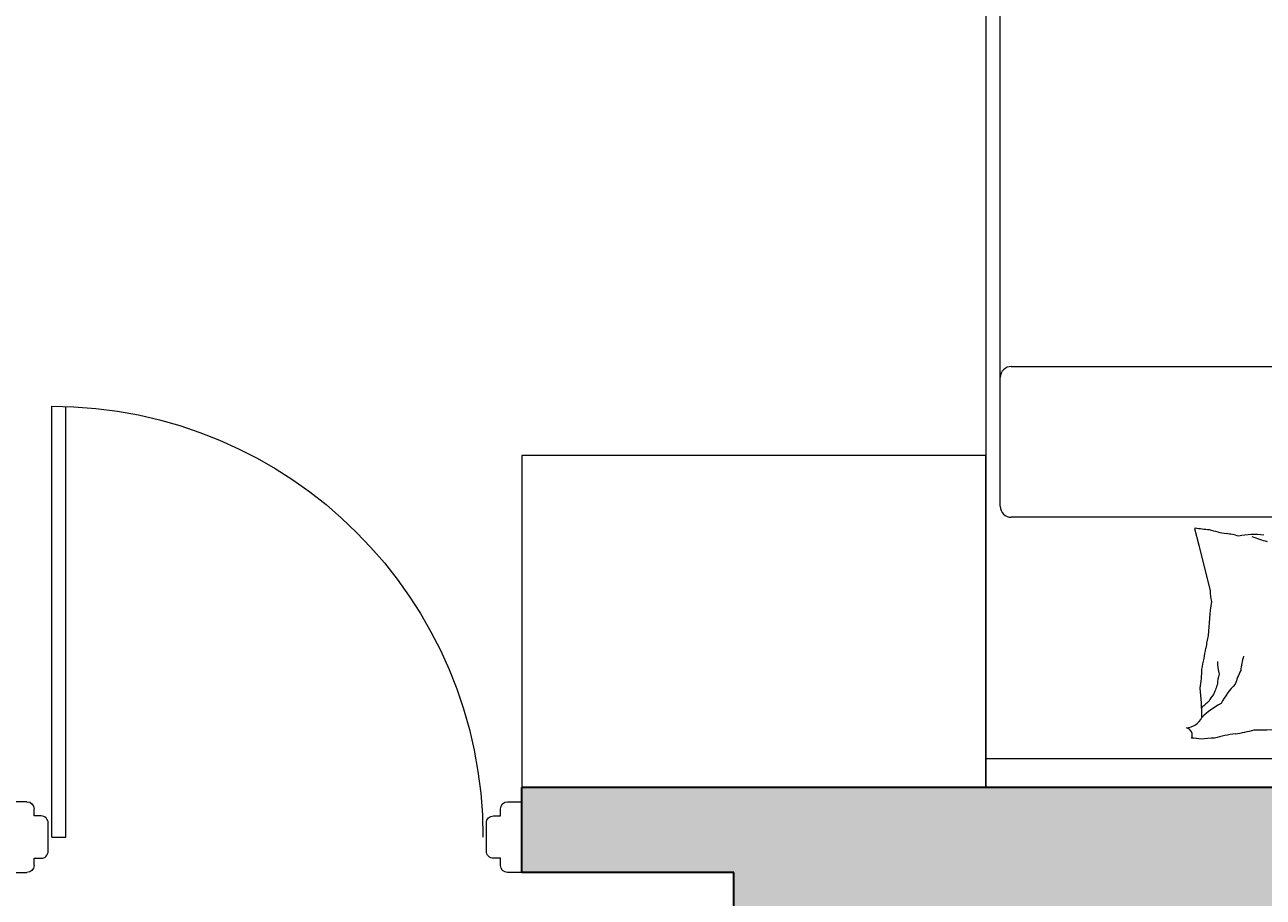
# Model space of a CAD drawing. Units: inches. Extents: x 84 to 1044, y -280 to 906.
# Tile 78 of 105: x 645 to 733, y 512 to 574. Entities that reach past the tile are written whole.
import ezdxf

# ---------------------------------------------------------------- set-up
doc = ezdxf.new("R2010")
doc.units = ezdxf.units.IN
for name, color, linetype, lineweight in [('00 FURNITURE', 15, 'Continuous', 15), ('A-ANNO-DIMS', 2, 'Continuous', 18), ('A-DOOR', 4, 'Continuous', 18), ('A-FURN', 8, 'Continuous', 15), ('WALL', 250, 'Continuous', 35)]:
    doc.layers.add(name, color=color, linetype=linetype, lineweight=lineweight)
doc.layers.add('A-WALL-PATT', color=251, linetype='Continuous', lineweight=9, true_color=0x636466)
doc.styles.get("Standard").update_dxf_attribs({"font": 'arial.ttf'})
doc.dimstyles.get("Standard").update_dxf_attribs({"dimtxt": 0.18, "dimasz": 0.18, "dimexe": 0.18, "dimexo": 0.0625, "dimgap": 0.09, "dimtad": 0, "dimtih": 1, "dimtoh": 1, "dimdec": 4, "dimzin": 0, "dimdsep": 46, "dimtxsty": 'Standard', "dimcen": 0.09, "dimadec": 0, "dimazin": 0, "dimtfac": 1, "dimtdec": 4, "dimtofl": 0, "dimtmove": 0, "dimatfit": 3, "dimfxl": 1, "dimtolj": 1, "dimtzin": 0, "dimarcsym": 0})

# ---------------------------------------------------------------- blocks, each defined once
blk = doc.blocks.new('DDD')
at = {"layer": '00 FURNITURE'}
for p, q in [((-12579.773, -15859.529), (-12579.773, -15829.045)), ((-12578.773, -15859.529), (-12578.773, -15829.029)), ((-12612.023, -15857.029), (-12612.023, -15862.029)), ((-12611.023, -15857.029), (-12612.023, -15857.029)), ((-12577.023, -15857.029), (-12576.023, -15857.029)), ((-12576.023, -15857.029), (-12576.023, -15862.029)), ((-12610.523, -15858.029), (-12610.523, -15857.529)), ((-12577.523, -15858.029), (-12577.523, -15857.529)), ((-12578.773, -15859.529), (-12579.773, -15859.529)), ((-12610.523, -15861.529), (-12610.523, -15861.029)), ((-12577.523, -15861.529), (-12577.523, -15861.029)), ((-12612.023, -15862.029), (-12611.023, -15862.029)), ((-12576.023, -15862.029), (-12577.023, -15862.029))]:
    blk.add_line(p, q, dxfattribs=at)
for points in [[(-12610.523, -15861.029), (-12610.023, -15861.029, 0.414214), (-12609.523, -15860.529), (-12609.523, -15858.529, 0.414214), (-12610.023, -15858.029), (-12610.523, -15858.029)], [(-12577.523, -15861.029), (-12578.023, -15861.029, -0.414214), (-12578.523, -15860.529), (-12578.523, -15858.529, -0.414214), (-12578.023, -15858.029), (-12577.523, -15858.029)]]:
    blk.add_lwpolyline(points, format="xyb", dxfattribs=at)
for centre, radius, start, end in [((-12578.773, -15859.529), 30.5, 90, 180), ((-12611.023, -15857.529), 0.5, 0, 90), ((-12577.023, -15857.529), 0.5, 90, 180), ((-12611.023, -15861.529), 0.5, 270, 0), ((-12577.023, -15861.529), 0.5, 180, 270)]:
    blk.add_arc(centre, radius, start, end, dxfattribs=at)
blk = doc.blocks.new('BED-DOUBLE-NIGHTSTANDS')
for p, q in [((33.845, 19.919), (33.845, 77.08)), ((34.629, 29.814), (88.271, 29.814)), ((85.85, 19.136), (34.629, 19.136)), ((47.596, 18.345), (47.89, 17.169)), ((47.89, 17.169), (48.699, 13.934)), ((32.834, 2.051), (111.174, 2.051))]:
    blk.add_line(p, q)
for points in [[(32.834, 78.34), (32.834, 0), (111.174, 0), (111.174, 78.34)], [(0.004, 23.502), (0.004, 0), (32.834, 0), (32.834, 23.502)]]:
    blk.add_lwpolyline(points, close=True)
for centre, radius, start, end in [((34.629, 29.03), 0.783, 90, 180), ((34.629, 19.919), 0.783, 180, 270), ((47.598, 18.38), 0.0359, 265.91706, 14.04494), ((49.381, 28.85), 10.605, 260.5159, 265.91706), ((51.314, 26.856), 8.996, 252.61359, 260.5159), ((49.306, 13.323), 4.69, 72.61359, 83.56595), ((51.852, 12.199), 5.715, 83.56595, 101.55856), ((61.275, 45.057), 28.934, 250.57202, 252.80178), ((74.329, 9.574), 25.804, 171.99495, 177.33512), ((51.349, 13.811), 2.652, 177.33512, 194.04519), ((60.693, 8.149), 12.422, 167.80162, 171.99495), ((14.336, 15.691), 34.549, 347.80162, 350.31563), ((52.799, 8.936), 3.585, 180, 194.68511), ((56.308, 7.745), 5.482, 163.48502, 174.36887), ((40.115, 8.39), 7.99, 350.31563, 0), ((51.414, 7.319), 2.2, 161.2201, 180), ((55.72, 5.76), 5.482, 152.60117, 163.48502), ((28.84, 4.955), 19.265, 0, 6.23236), ((56.689, 4.327), 8.052, 158.18508, 161.2201), ((54.334, 3.436), 5.482, 134.90238, 152.60117), ((50.464, 5.22), 2.061, 138.55709, 154.64488), ((54.414, 4.384), 5.918, 154.64488, 158.18508), ((50.684, 3.264), 3.52, 126.26407, 138.55709), ((51.973, 1.083), 5.482, 117.20359, 134.90238), ((46.913, 5.566), 1.339, 274.40021, 333.41948), ((46.915, 3.726), 0.514, 333.41948, 78.72762), ((52.232, -7.993), 11.938, 98.43719, 105.74398), ((49.235, 13.221), 9.489, 277.54685, 285.74398), ((51.809, 30.83), 26.741, 270, 277.54685), ((47.375, -0.045), 3.541, 78.72762, 90), ((48.993, -2.815), 6.312, 90, 98.43719)]:
    blk.add_arc(centre, radius, start, end)
blk = doc.blocks.new('*D62')
at = {"layer": 'A-ANNO-DIMS', "color": 0, "lineweight": -2, "transparency": 16777216}
for p, q in [((203.179, 709.183), (203.179, 905.9)), ((896.074, 400.183), (896.074, 905.9)), ((203.359, 905.72), (549.232, 905.72)), ((895.894, 905.72), (550.021, 905.72))]:
    blk.add_line(p, q, dxfattribs=at)
at = {"layer": 'A-ANNO-DIMS', "color": 0, "transparency": 16777216}
for points in [[(203.359, 905.75), (203.359, 905.69), (203.179, 905.72)], [(895.894, 905.75), (895.894, 905.69), (896.074, 905.72)]]:
    blk.add_solid(points, dxfattribs=at)
at = {"layer": 'Defpoints', "color": 0, "transparency": 16777216}
for p in [(896.074, 905.72), (203.179, 709.12), (896.074, 400.12)]:
    blk.add_point(p, dxfattribs=at)
at = {"layer": 'A-ANNO-DIMS', "color": 0, "transparency": 16777216, "insert": (549.627, 905.72), "char_height": 0.18, "attachment_point": 5}
blk.add_mtext('\\A1;692.9', dxfattribs=at)

msp = doc.modelspace()

# ---------------------------------------------------------------- hatches: boundary and pattern name
at = {"layer": 'A-WALL-PATT', "transparency": 33554597}
h = msp.add_hatch(color=256, dxfattribs=at)
h.dxf.hatch_style = 1
h.paths.add_polyline_path([(671.074, 100.12), (647.074, 100.12), (647.074, 160.12), (641.074, 160.12), (620.824, 160.12), (620.824, 151.12), (638.074, 151.12), (638.074, 91.12), (671.074, 91.12)])
h.paths.add_polyline_path([(791.074, 100.12), (743.074, 100.12), (743.074, 91.12), (791.074, 91.12)])
h.paths.add_polyline_path([(896.074, 346.12), (887.074, 346.12), (887.074, 334.12), (870.955, 334.12), (833.074, 334.12), (804.574, 334.12), (804.574, 328.12), (887.074, 328.12), (887.074, 100.12), (863.074, 100.12), (863.074, 91.12), (896.074, 91.12)])
h.paths.add_polyline_path([(507.574, 154.729), (507.574, 160.12), (464.074, 160.12), (464.074, 247.12), (641.074, 247.12), (641.074, 208.12), (647.074, 208.12), (647.074, 328.12), (659.074, 328.12), (659.074, 334.12), (617.074, 334.12), (617.074, 328.12), (641.074, 328.12), (641.074, 256.12), (545.074, 256.12), (545.074, 328.12), (569.074, 328.12), (569.074, 334.12), (518.074, 334.12), (518.074, 325.12), (536.074, 325.12), (536.074, 256.12), (464.074, 256.12), (464.074, 325.12), (482.074, 325.12), (482.074, 334.12), (455.074, 334.12), (455.074, 160.12), (413.127, 160.12), (413.127, 151.12), (455.074, 151.12), (455.074, 91.12), (464.074, 91.12), (464.074, 151.12), (507.574, 151.12)])
h.paths.add_polyline_path([(572.824, 160.12), (555.574, 160.12), (555.574, 151.12), (572.824, 151.12)], flags=17)
h.paths.add_polyline_path([(341.127, 160.12), (299.179, 160.12), (299.179, 211.12), (294.179, 211.12), (290.179, 211.12), (290.179, 151.12), (341.127, 151.12)])
h.paths.add_polyline_path([(299.179, 256.12), (212.179, 256.12), (212.179, 274.12), (203.179, 274.12), (203.179, 247.12), (299.179, 247.12)])
h.paths.add_polyline_path([(212.179, 514.12), (398.074, 514.12), (398.074, 519.12), (398.074, 520.12), (212.179, 520.12), (212.179, 574.12), (203.179, 574.12), (203.179, 310.12), (212.179, 310.12), (212.179, 328.12), (290.179, 328.12), (290.179, 292.12), (299.179, 292.12), (299.179, 328.12), (332.179, 328.12), (332.179, 334.12), (212.179, 334.12)])
h.paths.add_polyline_path([(287.127, 709.12), (203.179, 709.12), (203.179, 646.12), (212.179, 646.12), (212.179, 700.12), (287.127, 700.12)])
h.paths.add_polyline_path([(470.074, 709.12), (359.127, 709.12), (359.127, 700.12), (434.074, 700.12), (434.074, 574.12), (440.074, 574.12), (440.074, 622.12), (464.074, 622.12), (464.074, 628.12), (440.074, 628.12), (440.074, 700.12), (470.074, 700.12)])
h.paths.add_polyline_path([(572.074, 709.12), (506.074, 709.12), (506.074, 700.12), (536.074, 700.12), (536.074, 628.12), (494.074, 628.12), (494.074, 622.12), (536.074, 622.12), (536.074, 520.12), (440.074, 520.12), (440.074, 544.12), (434.074, 544.12), (434.074, 514.12), (644.074, 514.12), (644.074, 519.12), (644.074, 544.12), (638.074, 544.12), (638.074, 520.12), (542.074, 520.12), (542.074, 622.12), (584.074, 622.12), (584.074, 628.12), (542.074, 628.12), (542.074, 700.12), (572.074, 700.12)])
h.paths.add_polyline_path([(698.074, 709.12), (608.074, 709.12), (608.074, 700.12), (638.074, 700.12), (638.074, 628.12), (614.074, 628.12), (614.074, 622.12), (638.074, 622.12), (638.074, 574.12), (644.074, 574.12), (644.074, 700.12), (698.074, 700.12)])
h.paths.add_polyline_path([(833.074, 709.12), (770.074, 709.12), (770.074, 700.12), (824.074, 700.12), (824.074, 646.12), (833.074, 646.12)])
h.paths.add_polyline_path([(833.074, 574.12), (824.074, 574.12), (824.074, 520.12), (791.244, 520.12), (712.904, 520.12), (680.074, 520.12), (680.074, 514.12), (695.074, 514.12), (695.074, 491.62), (704.074, 491.62), (704.074, 511.12), (833.074, 511.12)])
h.paths.add_polyline_path([(704.074, 419.62), (695.074, 419.62), (695.074, 370.12), (704.074, 370.12)])
h.paths.add_polyline_path([(896.074, 400.12), (833.074, 400.12), (833.074, 364.12), (839.074, 364.12), (839.074, 394.12), (887.074, 394.12), (887.074, 382.12), (896.074, 382.12)])
h.paths.add_polyline_path([(732.574, 334.12), (695.074, 334.12), (695.074, 328.12), (732.574, 328.12)])

# ---------------------------------------------------------------- linework, layer by layer
at = {"layer": 'WALL'}
for p, q in [((680.074, 514.12), (680.074, 520.12)), ((824.074, 520.12), (680.074, 520.12)), ((695.074, 514.12), (680.074, 514.12)), ((695.074, 491.62), (695.074, 514.12))]:
    msp.add_line(p, q, dxfattribs=at)

# ---------------------------------------------------------------- block references
at = {"layer": 'A-DOOR', "xscale": -1}
msp.add_blockref('DDD', (-11931.95, 16376.149), dxfattribs=at)
at = {"layer": 'A-FURN'}
msp.add_blockref('BED-DOUBLE-NIGHTSTANDS', (680.07, 520.12), dxfattribs=at)

# ---------------------------------------------------------------- dimensions: what is measured, and where the dimension line sits
at = {"layer": 'A-ANNO-DIMS'}
dim = msp.add_linear_dim(base=(896.074, 905.72), p1=(203.179, 709.12), p2=(896.074, 400.12), dimstyle='Standard', override={"dimdec": 1, "dimlfac": 1, "dimrnd": 0, "dimzin": 0, "dimdsep": 46, "dimlunit": 2}, dxfattribs=at)
dim.commit()
dim.dimension.update_dxf_attribs({"geometry": '*D62', "text_midpoint": (549.627, 905.72)})

doc.saveas('drawing.dxf')
